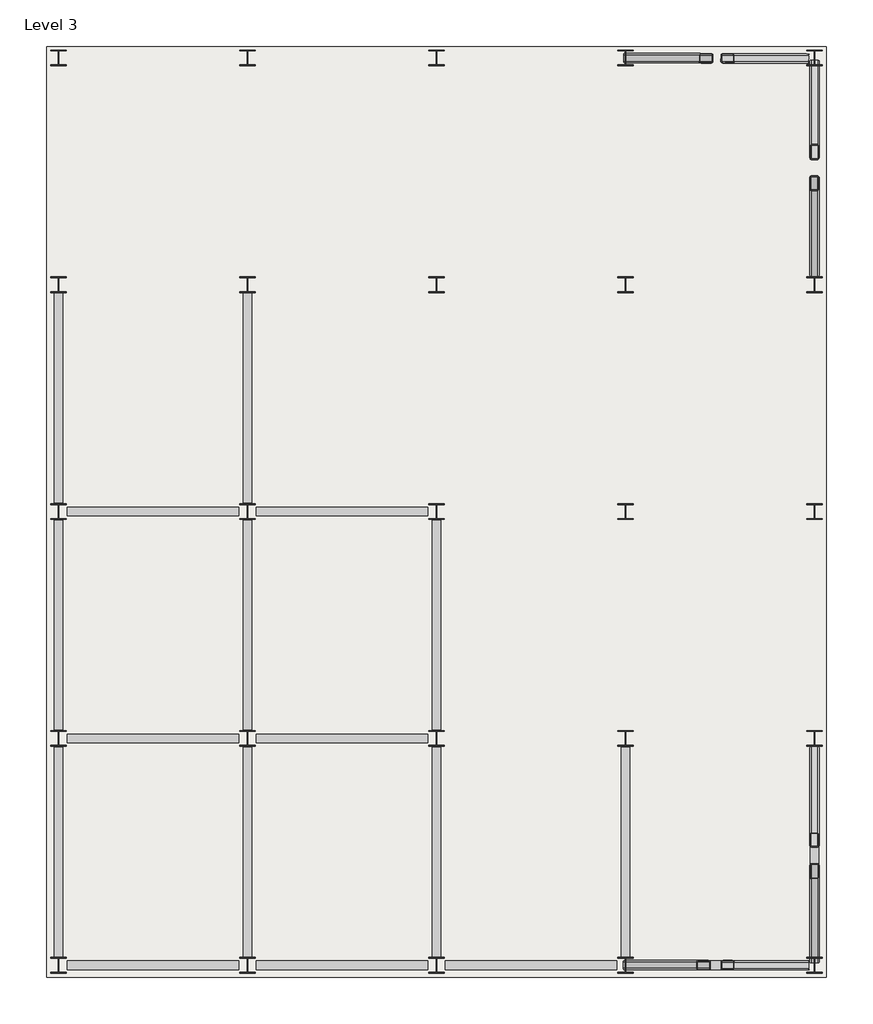
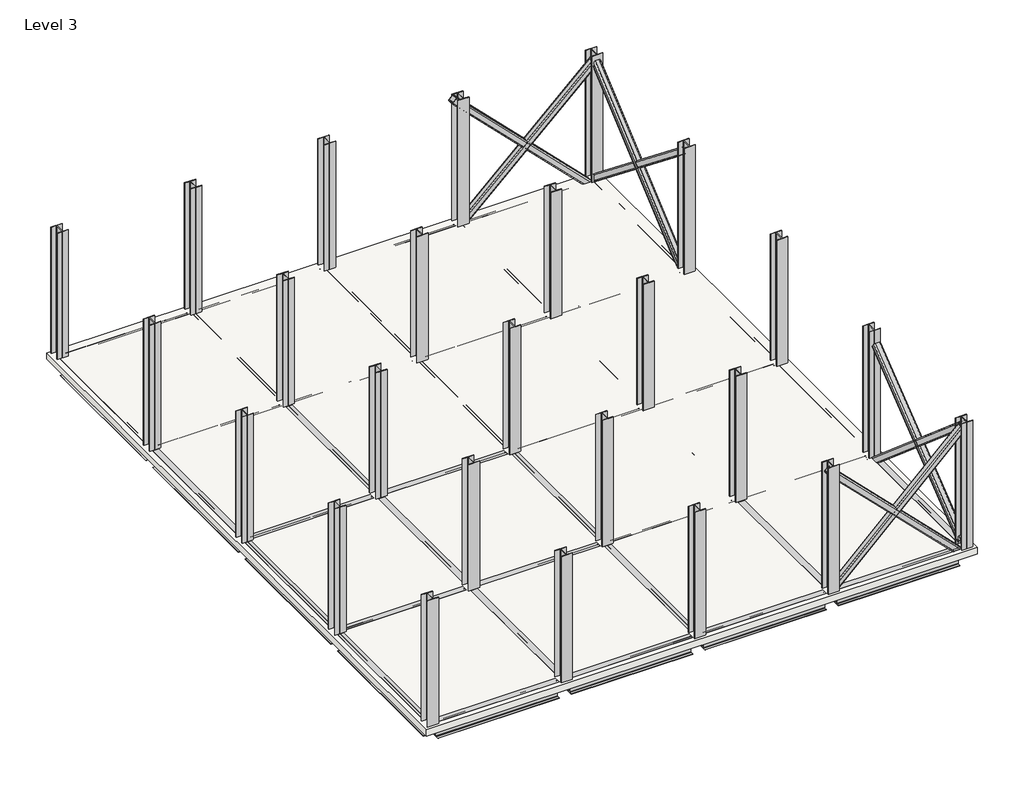
# One storey: 40 beams, 25 columns, 8 members, 1 slab.
"""IFC4 building model written with IfcOpenShell, lengths in millimetres."""

from ifc_helpers import new_model, si_unit, frame, origin, place, context, project, spatial, polyline, outline, extrude, transform, mapped, element, save
from components import w_shapes_w16x26_71b85d0e, w_shapes_w16x26_5730d789, w_shapes_column_w10x49_c7b378f5, hss_square_hss6x6x1_2_008024fe, hss_square_hss6x6x1_2_7c43692b, hss_square_hss6x6x1_2_5f011b37, hss_square_hss6x6x1_2_b9926e2d, hss_square_hss6x6x1_2_e6555cf9, hss_square_hss6x6x1_2_f7a49a43, hss_square_hss6x6x1_2_10b7330d, hss_square_hss6x6x1_2_f3b36863

model = new_model("IFC4")

# Units and contexts
model_context = context("Model", 3, world=origin())
ifc_project = project(units=[si_unit("LENGTHUNIT", "METRE", prefix="MILLI")], contexts=[model_context])

# Site, building, storey
site = spatial("IfcSite", under=ifc_project)
building = spatial("IfcBuilding", under=site)
storey = spatial("IfcBuildingStorey", under=building, Name="Level 3", Elevation=6096.0)

# Beams
placement = place(None, origin())
w_shapes_w16x26_shape = w_shapes_w16x26_71b85d0e(model_context)
element("IfcBeam", 1, ObjectType="W Shapes : W16X26", at=placement, inside=storey, context=model_context, shape_type="MappedRepresentation", body=[
    mapped(w_shapes_w16x26_shape, transform((-5883.5186598, -2213.7239423, 5896.61), x_axis=(1.0, 0.0, 0.0), y_axis=(0.0, 1.0, 0.0), z_axis=(0.0, 0.0, 1.0))),
])
element("IfcBeam", 2, ObjectType="W Shapes : W16X26", at=placement, inside=storey, context=model_context, shape_type="MappedRepresentation", body=[
    mapped(w_shapes_w16x26_shape, transform((-2835.5186598, -2213.7239423, 5896.61), x_axis=(1.0, 0.0, 0.0), y_axis=(0.0, 1.0, 0.0), z_axis=(0.0, 0.0, 1.0))),
])
element("IfcBeam", 3, ObjectType="W Shapes : W16X26", at=placement, inside=storey, context=model_context, shape_type="MappedRepresentation", body=[
    mapped(w_shapes_w16x26_shape, transform((212.4813402, -2213.7239423, 5896.61), x_axis=(1.0, 0.0, 0.0), y_axis=(0.0, 1.0, 0.0), z_axis=(0.0, 0.0, 1.0))),
])
element("IfcBeam", 4, ObjectType="W Shapes : W16X26", at=placement, inside=storey, context=model_context, shape_type="MappedRepresentation", body=[
    mapped(w_shapes_w16x26_shape, transform((3260.4813402, -2213.7239423, 5896.61), x_axis=(1.0, 0.0, 0.0), y_axis=(0.0, 1.0, 0.0), z_axis=(0.0, 0.0, 1.0))),
])
element("IfcBeam", 5, ObjectType="W Shapes : W16X26", at=placement, inside=storey, context=model_context, shape_type="MappedRepresentation", body=[
    mapped(w_shapes_w16x26_shape, transform((-5883.5186598, 1443.8760577, 5896.61), x_axis=(1.0, 0.0, 0.0), y_axis=(0.0, 1.0, 0.0), z_axis=(0.0, 0.0, 1.0))),
])
element("IfcBeam", 6, ObjectType="W Shapes : W16X26", at=placement, inside=storey, context=model_context, shape_type="MappedRepresentation", body=[
    mapped(w_shapes_w16x26_shape, transform((-2835.5186598, 1443.8760577, 5896.61), x_axis=(1.0, 0.0, 0.0), y_axis=(0.0, 1.0, 0.0), z_axis=(0.0, 0.0, 1.0))),
])
element("IfcBeam", 7, ObjectType="W Shapes : W16X26", at=placement, inside=storey, context=model_context, shape_type="MappedRepresentation", body=[
    mapped(w_shapes_w16x26_shape, transform((212.4813402, 1443.8760577, 5896.61), x_axis=(1.0, 0.0, 0.0), y_axis=(0.0, 1.0, 0.0), z_axis=(0.0, 0.0, 1.0))),
])
element("IfcBeam", 8, ObjectType="W Shapes : W16X26", at=placement, inside=storey, context=model_context, shape_type="MappedRepresentation", body=[
    mapped(w_shapes_w16x26_shape, transform((3260.4813402, 1443.8760577, 5896.61), x_axis=(1.0, 0.0, 0.0), y_axis=(0.0, 1.0, 0.0), z_axis=(0.0, 0.0, 1.0))),
])
element("IfcBeam", 9, ObjectType="W Shapes : W16X26", at=placement, inside=storey, context=model_context, shape_type="MappedRepresentation", body=[
    mapped(w_shapes_w16x26_shape, transform((-5883.5186598, 5101.4760577, 5896.61), x_axis=(1.0, 0.0, 0.0), y_axis=(0.0, 1.0, 0.0), z_axis=(0.0, 0.0, 1.0))),
])
element("IfcBeam", 10, ObjectType="W Shapes : W16X26", at=placement, inside=storey, context=model_context, shape_type="MappedRepresentation", body=[
    mapped(w_shapes_w16x26_shape, transform((-2835.5186598, 5101.4760577, 5896.61), x_axis=(1.0, 0.0, 0.0), y_axis=(0.0, 1.0, 0.0), z_axis=(0.0, 0.0, 1.0))),
])
element("IfcBeam", 11, ObjectType="W Shapes : W16X26", at=placement, inside=storey, context=model_context, shape_type="MappedRepresentation", body=[
    mapped(w_shapes_w16x26_shape, transform((212.4813402, 5101.4760577, 5896.61), x_axis=(1.0, 0.0, 0.0), y_axis=(0.0, 1.0, 0.0), z_axis=(0.0, 0.0, 1.0))),
])
element("IfcBeam", 12, ObjectType="W Shapes : W16X26", at=placement, inside=storey, context=model_context, shape_type="MappedRepresentation", body=[
    mapped(w_shapes_w16x26_shape, transform((3260.4813402, 5101.4760577, 5896.61), x_axis=(1.0, 0.0, 0.0), y_axis=(0.0, 1.0, 0.0), z_axis=(0.0, 0.0, 1.0))),
])
element("IfcBeam", 13, ObjectType="W Shapes : W16X26", at=placement, inside=storey, context=model_context, shape_type="MappedRepresentation", body=[
    mapped(w_shapes_w16x26_shape, transform((-5883.5186598, 8759.0760577, 5896.61), x_axis=(1.0, 0.0, 0.0), y_axis=(0.0, 1.0, 0.0), z_axis=(0.0, 0.0, 1.0))),
])
element("IfcBeam", 14, ObjectType="W Shapes : W16X26", at=placement, inside=storey, context=model_context, shape_type="MappedRepresentation", body=[
    mapped(w_shapes_w16x26_shape, transform((-2835.5186598, 8759.0760577, 5896.61), x_axis=(1.0, 0.0, 0.0), y_axis=(0.0, 1.0, 0.0), z_axis=(0.0, 0.0, 1.0))),
])
element("IfcBeam", 15, ObjectType="W Shapes : W16X26", at=placement, inside=storey, context=model_context, shape_type="MappedRepresentation", body=[
    mapped(w_shapes_w16x26_shape, transform((212.4813402, 8759.0760577, 5896.61), x_axis=(1.0, 0.0, 0.0), y_axis=(0.0, 1.0, 0.0), z_axis=(0.0, 0.0, 1.0))),
])
element("IfcBeam", 16, ObjectType="W Shapes : W16X26", at=placement, inside=storey, context=model_context, shape_type="MappedRepresentation", body=[
    mapped(w_shapes_w16x26_shape, transform((3260.4813402, 8759.0760577, 5896.61), x_axis=(1.0, 0.0, 0.0), y_axis=(0.0, 1.0, 0.0), z_axis=(0.0, 0.0, 1.0))),
])
element("IfcBeam", 17, ObjectType="W Shapes : W16X26", at=placement, inside=storey, context=model_context, shape_type="MappedRepresentation", body=[
    mapped(w_shapes_w16x26_shape, transform((-5883.5186598, 12416.6760577, 5896.61), x_axis=(1.0, 0.0, 0.0), y_axis=(0.0, 1.0, 0.0), z_axis=(0.0, 0.0, 1.0))),
])
element("IfcBeam", 18, ObjectType="W Shapes : W16X26", at=placement, inside=storey, context=model_context, shape_type="MappedRepresentation", body=[
    mapped(w_shapes_w16x26_shape, transform((-2835.5186598, 12416.6760577, 5896.61), x_axis=(1.0, 0.0, 0.0), y_axis=(0.0, 1.0, 0.0), z_axis=(0.0, 0.0, 1.0))),
])
element("IfcBeam", 19, ObjectType="W Shapes : W16X26", at=placement, inside=storey, context=model_context, shape_type="MappedRepresentation", body=[
    mapped(w_shapes_w16x26_shape, transform((212.4813402, 12416.6760577, 5896.61), x_axis=(1.0, 0.0, 0.0), y_axis=(0.0, 1.0, 0.0), z_axis=(0.0, 0.0, 1.0))),
])
element("IfcBeam", 20, ObjectType="W Shapes : W16X26", at=placement, inside=storey, context=model_context, shape_type="MappedRepresentation", body=[
    mapped(w_shapes_w16x26_shape, transform((3260.4813402, 12416.6760577, 5896.61), x_axis=(1.0, 0.0, 0.0), y_axis=(0.0, 1.0, 0.0), z_axis=(0.0, 0.0, 1.0))),
])
w_shapes_w16x26_2_shape = w_shapes_w16x26_5730d789(model_context)
element("IfcBeam", 21, ObjectType="W Shapes : W16X26", at=placement, inside=storey, context=model_context, shape_type="MappedRepresentation", body=[
    mapped(w_shapes_w16x26_2_shape, transform((4784.4813402, 10587.8760577, 5896.61), x_axis=(0.0, -1.0, 0.0), y_axis=(1.0, 0.0, 0.0), z_axis=(0.0, 0.0, 1.0))),
])
element("IfcBeam", 22, ObjectType="W Shapes : W16X26", at=placement, inside=storey, context=model_context, shape_type="MappedRepresentation", body=[
    mapped(w_shapes_w16x26_2_shape, transform((4784.4813402, 6930.2760577, 5896.61), x_axis=(0.0, -1.0, 0.0), y_axis=(1.0, 0.0, 0.0), z_axis=(0.0, 0.0, 1.0))),
])
element("IfcBeam", 23, ObjectType="W Shapes : W16X26", at=placement, inside=storey, context=model_context, shape_type="MappedRepresentation", body=[
    mapped(w_shapes_w16x26_2_shape, transform((4784.4813402, 3272.6760577, 5896.61), x_axis=(0.0, -1.0, 0.0), y_axis=(1.0, 0.0, 0.0), z_axis=(0.0, 0.0, 1.0))),
])
element("IfcBeam", 24, ObjectType="W Shapes : W16X26", at=placement, inside=storey, context=model_context, shape_type="MappedRepresentation", body=[
    mapped(w_shapes_w16x26_2_shape, transform((4784.4813402, -384.9239423, 5896.61), x_axis=(0.0, -1.0, 0.0), y_axis=(1.0, 0.0, 0.0), z_axis=(0.0, 0.0, 1.0))),
])
element("IfcBeam", 25, ObjectType="W Shapes : W16X26", at=placement, inside=storey, context=model_context, shape_type="MappedRepresentation", body=[
    mapped(w_shapes_w16x26_2_shape, transform((1736.4813402, 10587.8760577, 5896.61), x_axis=(0.0, -1.0, 0.0), y_axis=(1.0, 0.0, 0.0), z_axis=(0.0, 0.0, 1.0))),
])
element("IfcBeam", 26, ObjectType="W Shapes : W16X26", at=placement, inside=storey, context=model_context, shape_type="MappedRepresentation", body=[
    mapped(w_shapes_w16x26_2_shape, transform((1736.4813402, 6930.2760577, 5896.61), x_axis=(0.0, -1.0, 0.0), y_axis=(1.0, 0.0, 0.0), z_axis=(0.0, 0.0, 1.0))),
])
element("IfcBeam", 27, ObjectType="W Shapes : W16X26", at=placement, inside=storey, context=model_context, shape_type="MappedRepresentation", body=[
    mapped(w_shapes_w16x26_2_shape, transform((1736.4813402, 3272.6760577, 5896.61), x_axis=(0.0, -1.0, 0.0), y_axis=(1.0, 0.0, 0.0), z_axis=(0.0, 0.0, 1.0))),
])
element("IfcBeam", 28, ObjectType="W Shapes : W16X26", at=placement, inside=storey, context=model_context, shape_type="MappedRepresentation", body=[
    mapped(w_shapes_w16x26_2_shape, transform((1736.4813402, -384.9239423, 5896.61), x_axis=(0.0, -1.0, 0.0), y_axis=(1.0, 0.0, 0.0), z_axis=(0.0, 0.0, 1.0))),
])
element("IfcBeam", 29, ObjectType="W Shapes : W16X26", at=placement, inside=storey, context=model_context, shape_type="MappedRepresentation", body=[
    mapped(w_shapes_w16x26_2_shape, transform((-1311.5186598, 10587.8760577, 5896.61), x_axis=(0.0, -1.0, 0.0), y_axis=(1.0, 0.0, 0.0), z_axis=(0.0, 0.0, 1.0))),
])
element("IfcBeam", 30, ObjectType="W Shapes : W16X26", at=placement, inside=storey, context=model_context, shape_type="MappedRepresentation", body=[
    mapped(w_shapes_w16x26_2_shape, transform((-1311.5186598, 6930.2760577, 5896.61), x_axis=(0.0, -1.0, 0.0), y_axis=(1.0, 0.0, 0.0), z_axis=(0.0, 0.0, 1.0))),
])
element("IfcBeam", 31, ObjectType="W Shapes : W16X26", at=placement, inside=storey, context=model_context, shape_type="MappedRepresentation", body=[
    mapped(w_shapes_w16x26_2_shape, transform((-1311.5186598, 3272.6760577, 5896.61), x_axis=(0.0, -1.0, 0.0), y_axis=(1.0, 0.0, 0.0), z_axis=(0.0, 0.0, 1.0))),
])
element("IfcBeam", 32, ObjectType="W Shapes : W16X26", at=placement, inside=storey, context=model_context, shape_type="MappedRepresentation", body=[
    mapped(w_shapes_w16x26_2_shape, transform((-1311.5186598, -384.9239423, 5896.61), x_axis=(0.0, -1.0, 0.0), y_axis=(1.0, 0.0, 0.0), z_axis=(0.0, 0.0, 1.0))),
])
element("IfcBeam", 33, ObjectType="W Shapes : W16X26", at=placement, inside=storey, context=model_context, shape_type="MappedRepresentation", body=[
    mapped(w_shapes_w16x26_2_shape, transform((-4359.5186598, 10587.8760577, 5896.61), x_axis=(0.0, -1.0, 0.0), y_axis=(1.0, 0.0, 0.0), z_axis=(0.0, 0.0, 1.0))),
])
element("IfcBeam", 34, ObjectType="W Shapes : W16X26", at=placement, inside=storey, context=model_context, shape_type="MappedRepresentation", body=[
    mapped(w_shapes_w16x26_2_shape, transform((-4359.5186598, 6930.2760577, 5896.61), x_axis=(0.0, -1.0, 0.0), y_axis=(1.0, 0.0, 0.0), z_axis=(0.0, 0.0, 1.0))),
])
element("IfcBeam", 35, ObjectType="W Shapes : W16X26", at=placement, inside=storey, context=model_context, shape_type="MappedRepresentation", body=[
    mapped(w_shapes_w16x26_2_shape, transform((-4359.5186598, 3272.6760577, 5896.61), x_axis=(0.0, -1.0, 0.0), y_axis=(1.0, 0.0, 0.0), z_axis=(0.0, 0.0, 1.0))),
])
element("IfcBeam", 36, ObjectType="W Shapes : W16X26", at=placement, inside=storey, context=model_context, shape_type="MappedRepresentation", body=[
    mapped(w_shapes_w16x26_2_shape, transform((-4359.5186598, -384.9239423, 5896.61), x_axis=(0.0, -1.0, 0.0), y_axis=(1.0, 0.0, 0.0), z_axis=(0.0, 0.0, 1.0))),
])
element("IfcBeam", 37, ObjectType="W Shapes : W16X26", at=placement, inside=storey, context=model_context, shape_type="MappedRepresentation", body=[
    mapped(w_shapes_w16x26_2_shape, transform((-7407.5186598, 10587.8760577, 5896.61), x_axis=(0.0, -1.0, 0.0), y_axis=(1.0, 0.0, 0.0), z_axis=(0.0, 0.0, 1.0))),
])
element("IfcBeam", 38, ObjectType="W Shapes : W16X26", at=placement, inside=storey, context=model_context, shape_type="MappedRepresentation", body=[
    mapped(w_shapes_w16x26_2_shape, transform((-7407.5186598, 6930.2760577, 5896.61), x_axis=(0.0, -1.0, 0.0), y_axis=(1.0, 0.0, 0.0), z_axis=(0.0, 0.0, 1.0))),
])
element("IfcBeam", 39, ObjectType="W Shapes : W16X26", at=placement, inside=storey, context=model_context, shape_type="MappedRepresentation", body=[
    mapped(w_shapes_w16x26_2_shape, transform((-7407.5186598, 3272.6760577, 5896.61), x_axis=(0.0, -1.0, 0.0), y_axis=(1.0, 0.0, 0.0), z_axis=(0.0, 0.0, 1.0))),
])
element("IfcBeam", 40, ObjectType="W Shapes : W16X26", at=placement, inside=storey, context=model_context, shape_type="MappedRepresentation", body=[
    mapped(w_shapes_w16x26_2_shape, transform((-7407.5186598, -384.9239423, 5896.61), x_axis=(0.0, -1.0, 0.0), y_axis=(1.0, 0.0, 0.0), z_axis=(0.0, 0.0, 1.0))),
])

# Columns
w_shapes_column_w10x49_shape = w_shapes_column_w10x49_c7b378f5(model_context)
element("IfcColumn", 41, ObjectType="W Shapes-Column : W10X49", at=placement, inside=storey, context=model_context, shape_type="MappedRepresentation", body=[
    mapped(w_shapes_column_w10x49_shape, transform((4784.4813402, -2213.7239423, 0.0), x_axis=(1.0, 0.0, 0.0), y_axis=(0.0, 1.0, 0.0), z_axis=(0.0, 0.0, 1.0))),
])
element("IfcColumn", 42, ObjectType="W Shapes-Column : W10X49", at=placement, inside=storey, context=model_context, shape_type="MappedRepresentation", body=[
    mapped(w_shapes_column_w10x49_shape, transform((1736.4813402, -2213.7239423, 0.0), x_axis=(1.0, 0.0, 0.0), y_axis=(0.0, 1.0, 0.0), z_axis=(0.0, 0.0, 1.0))),
])
element("IfcColumn", 43, ObjectType="W Shapes-Column : W10X49", at=placement, inside=storey, context=model_context, shape_type="MappedRepresentation", body=[
    mapped(w_shapes_column_w10x49_shape, transform((-1311.5186598, -2213.7239423, 0.0), x_axis=(1.0, 0.0, 0.0), y_axis=(0.0, 1.0, 0.0), z_axis=(0.0, 0.0, 1.0))),
])
element("IfcColumn", 44, ObjectType="W Shapes-Column : W10X49", at=placement, inside=storey, context=model_context, shape_type="MappedRepresentation", body=[
    mapped(w_shapes_column_w10x49_shape, transform((-4359.5186598, -2213.7239423, 0.0), x_axis=(1.0, 0.0, 0.0), y_axis=(0.0, 1.0, 0.0), z_axis=(0.0, 0.0, 1.0))),
])
element("IfcColumn", 45, ObjectType="W Shapes-Column : W10X49", at=placement, inside=storey, context=model_context, shape_type="MappedRepresentation", body=[
    mapped(w_shapes_column_w10x49_shape, transform((-7407.5186598, -2213.7239423, 0.0), x_axis=(1.0, 0.0, 0.0), y_axis=(0.0, 1.0, 0.0), z_axis=(0.0, 0.0, 1.0))),
])
element("IfcColumn", 46, ObjectType="W Shapes-Column : W10X49", at=placement, inside=storey, context=model_context, shape_type="MappedRepresentation", body=[
    mapped(w_shapes_column_w10x49_shape, transform((4784.4813402, 1443.8760577, 0.0), x_axis=(1.0, 0.0, 0.0), y_axis=(0.0, 1.0, 0.0), z_axis=(0.0, 0.0, 1.0))),
])
element("IfcColumn", 47, ObjectType="W Shapes-Column : W10X49", at=placement, inside=storey, context=model_context, shape_type="MappedRepresentation", body=[
    mapped(w_shapes_column_w10x49_shape, transform((4784.4813402, 5101.4760577, 0.0), x_axis=(1.0, 0.0, 0.0), y_axis=(0.0, 1.0, 0.0), z_axis=(0.0, 0.0, 1.0))),
])
element("IfcColumn", 48, ObjectType="W Shapes-Column : W10X49", at=placement, inside=storey, context=model_context, shape_type="MappedRepresentation", body=[
    mapped(w_shapes_column_w10x49_shape, transform((4784.4813402, 8759.0760577, 0.0), x_axis=(1.0, 0.0, 0.0), y_axis=(0.0, 1.0, 0.0), z_axis=(0.0, 0.0, 1.0))),
])
element("IfcColumn", 49, ObjectType="W Shapes-Column : W10X49", at=placement, inside=storey, context=model_context, shape_type="MappedRepresentation", body=[
    mapped(w_shapes_column_w10x49_shape, transform((4784.4813402, 12416.6760577, 0.0), x_axis=(1.0, 0.0, 0.0), y_axis=(0.0, 1.0, 0.0), z_axis=(0.0, 0.0, 1.0))),
])
element("IfcColumn", 50, ObjectType="W Shapes-Column : W10X49", at=placement, inside=storey, context=model_context, shape_type="MappedRepresentation", body=[
    mapped(w_shapes_column_w10x49_shape, transform((1736.4813402, 1443.8760577, 0.0), x_axis=(1.0, 0.0, 0.0), y_axis=(0.0, 1.0, 0.0), z_axis=(0.0, 0.0, 1.0))),
])
element("IfcColumn", 51, ObjectType="W Shapes-Column : W10X49", at=placement, inside=storey, context=model_context, shape_type="MappedRepresentation", body=[
    mapped(w_shapes_column_w10x49_shape, transform((-1311.5186598, 1443.8760577, 0.0), x_axis=(1.0, 0.0, 0.0), y_axis=(0.0, 1.0, 0.0), z_axis=(0.0, 0.0, 1.0))),
])
element("IfcColumn", 52, ObjectType="W Shapes-Column : W10X49", at=placement, inside=storey, context=model_context, shape_type="MappedRepresentation", body=[
    mapped(w_shapes_column_w10x49_shape, transform((-4359.5186598, 1443.8760577, 0.0), x_axis=(1.0, 0.0, 0.0), y_axis=(0.0, 1.0, 0.0), z_axis=(0.0, 0.0, 1.0))),
])
element("IfcColumn", 53, ObjectType="W Shapes-Column : W10X49", at=placement, inside=storey, context=model_context, shape_type="MappedRepresentation", body=[
    mapped(w_shapes_column_w10x49_shape, transform((-7407.5186598, 1443.8760577, 0.0), x_axis=(1.0, 0.0, 0.0), y_axis=(0.0, 1.0, 0.0), z_axis=(0.0, 0.0, 1.0))),
])
element("IfcColumn", 54, ObjectType="W Shapes-Column : W10X49", at=placement, inside=storey, context=model_context, shape_type="MappedRepresentation", body=[
    mapped(w_shapes_column_w10x49_shape, transform((1736.4813402, 5101.4760577, 0.0), x_axis=(1.0, 0.0, 0.0), y_axis=(0.0, 1.0, 0.0), z_axis=(0.0, 0.0, 1.0))),
])
element("IfcColumn", 55, ObjectType="W Shapes-Column : W10X49", at=placement, inside=storey, context=model_context, shape_type="MappedRepresentation", body=[
    mapped(w_shapes_column_w10x49_shape, transform((-1311.5186598, 5101.4760577, 0.0), x_axis=(1.0, 0.0, 0.0), y_axis=(0.0, 1.0, 0.0), z_axis=(0.0, 0.0, 1.0))),
])
element("IfcColumn", 56, ObjectType="W Shapes-Column : W10X49", at=placement, inside=storey, context=model_context, shape_type="MappedRepresentation", body=[
    mapped(w_shapes_column_w10x49_shape, transform((-4359.5186598, 5101.4760577, 0.0), x_axis=(1.0, 0.0, 0.0), y_axis=(0.0, 1.0, 0.0), z_axis=(0.0, 0.0, 1.0))),
])
element("IfcColumn", 57, ObjectType="W Shapes-Column : W10X49", at=placement, inside=storey, context=model_context, shape_type="MappedRepresentation", body=[
    mapped(w_shapes_column_w10x49_shape, transform((-7407.5186598, 5101.4760577, 0.0), x_axis=(1.0, 0.0, 0.0), y_axis=(0.0, 1.0, 0.0), z_axis=(0.0, 0.0, 1.0))),
])
element("IfcColumn", 58, ObjectType="W Shapes-Column : W10X49", at=placement, inside=storey, context=model_context, shape_type="MappedRepresentation", body=[
    mapped(w_shapes_column_w10x49_shape, transform((1736.4813402, 8759.0760577, 0.0), x_axis=(1.0, 0.0, 0.0), y_axis=(0.0, 1.0, 0.0), z_axis=(0.0, 0.0, 1.0))),
])
element("IfcColumn", 59, ObjectType="W Shapes-Column : W10X49", at=placement, inside=storey, context=model_context, shape_type="MappedRepresentation", body=[
    mapped(w_shapes_column_w10x49_shape, transform((-1311.5186598, 8759.0760577, 0.0), x_axis=(1.0, 0.0, 0.0), y_axis=(0.0, 1.0, 0.0), z_axis=(0.0, 0.0, 1.0))),
])
element("IfcColumn", 60, ObjectType="W Shapes-Column : W10X49", at=placement, inside=storey, context=model_context, shape_type="MappedRepresentation", body=[
    mapped(w_shapes_column_w10x49_shape, transform((-4359.5186598, 8759.0760577, 0.0), x_axis=(1.0, 0.0, 0.0), y_axis=(0.0, 1.0, 0.0), z_axis=(0.0, 0.0, 1.0))),
])
element("IfcColumn", 61, ObjectType="W Shapes-Column : W10X49", at=placement, inside=storey, context=model_context, shape_type="MappedRepresentation", body=[
    mapped(w_shapes_column_w10x49_shape, transform((-7407.5186598, 8759.0760577, 0.0), x_axis=(1.0, 0.0, 0.0), y_axis=(0.0, 1.0, 0.0), z_axis=(0.0, 0.0, 1.0))),
])
element("IfcColumn", 62, ObjectType="W Shapes-Column : W10X49", at=placement, inside=storey, context=model_context, shape_type="MappedRepresentation", body=[
    mapped(w_shapes_column_w10x49_shape, transform((1736.4813402, 12416.6760577, 0.0), x_axis=(1.0, 0.0, 0.0), y_axis=(0.0, 1.0, 0.0), z_axis=(0.0, 0.0, 1.0))),
])
element("IfcColumn", 63, ObjectType="W Shapes-Column : W10X49", at=placement, inside=storey, context=model_context, shape_type="MappedRepresentation", body=[
    mapped(w_shapes_column_w10x49_shape, transform((-1311.5186598, 12416.6760577, 0.0), x_axis=(1.0, 0.0, 0.0), y_axis=(0.0, 1.0, 0.0), z_axis=(0.0, 0.0, 1.0))),
])
element("IfcColumn", 64, ObjectType="W Shapes-Column : W10X49", at=placement, inside=storey, context=model_context, shape_type="MappedRepresentation", body=[
    mapped(w_shapes_column_w10x49_shape, transform((-4359.5186598, 12416.6760577, 0.0), x_axis=(1.0, 0.0, 0.0), y_axis=(0.0, 1.0, 0.0), z_axis=(0.0, 0.0, 1.0))),
])
element("IfcColumn", 65, ObjectType="W Shapes-Column : W10X49", at=placement, inside=storey, context=model_context, shape_type="MappedRepresentation", body=[
    mapped(w_shapes_column_w10x49_shape, transform((-7407.5186598, 12416.6760577, 0.0), x_axis=(1.0, 0.0, 0.0), y_axis=(0.0, 1.0, 0.0), z_axis=(0.0, 0.0, 1.0))),
])

# Members
hss_square_hss6x6x1_2_shape = hss_square_hss6x6x1_2_008024fe(model_context)
element("IfcMember", 66, ObjectType="HSS Square : HSS6X6X1/2", at=placement, inside=storey, context=model_context, shape_type="MappedRepresentation", body=[
    mapped(hss_square_hss6x6x1_2_shape, transform((4784.4813402, 10587.8760577, 7543.8), x_axis=(0.0, 0.7840458244617616, -0.6207029443655613), y_axis=(-1.0000000000000002, 0.0, 0.0), z_axis=(0.0, 0.6207029443655613, 0.7840458244617616))),
])
hss_square_hss6x6x1_2_2_shape = hss_square_hss6x6x1_2_7c43692b(model_context)
element("IfcMember", 67, ObjectType="HSS Square : HSS6X6X1/2", at=placement, inside=storey, context=model_context, shape_type="MappedRepresentation", body=[
    mapped(hss_square_hss6x6x1_2_2_shape, transform((4784.4813402, 10587.8760577, 7460.1631022), x_axis=(0.0, -0.760075346032819, -0.6498349547024159), y_axis=(1.0000000000000002, 0.0, 0.0), z_axis=(0.0, -0.6498349547024159, 0.760075346032819))),
])
hss_square_hss6x6x1_2_3_shape = hss_square_hss6x6x1_2_5f011b37(model_context)
element("IfcMember", 68, ObjectType="HSS Square : HSS6X6X1/2", at=placement, inside=storey, context=model_context, shape_type="MappedRepresentation", body=[
    mapped(hss_square_hss6x6x1_2_3_shape, transform((4784.4813402, -384.9239423, 7460.1631022), x_axis=(0.0, 0.760075346032819, -0.6498349547024159), y_axis=(-1.0000000000000002, 0.0, 0.0), z_axis=(0.0, 0.6498349547024159, 0.760075346032819))),
])
hss_square_hss6x6x1_2_4_shape = hss_square_hss6x6x1_2_b9926e2d(model_context)
element("IfcMember", 69, ObjectType="HSS Square : HSS6X6X1/2", at=placement, inside=storey, context=model_context, shape_type="MappedRepresentation", body=[
    mapped(hss_square_hss6x6x1_2_4_shape, transform((4784.4813402, -384.9239423, 7543.8), x_axis=(0.0, -0.7840458244617616, -0.6207029443655613), y_axis=(1.0000000000000002, 0.0, 0.0), z_axis=(0.0, -0.6207029443655613, 0.7840458244617616))),
])
hss_square_hss6x6x1_2_5_shape = hss_square_hss6x6x1_2_e6555cf9(model_context)
element("IfcMember", 70, ObjectType="HSS Square : HSS6X6X1/2", at=placement, inside=storey, context=model_context, shape_type="MappedRepresentation", body=[
    mapped(hss_square_hss6x6x1_2_5_shape, transform((3168.0352384, -2213.7239423, 7461.8521986), x_axis=(-0.718393447364439, 0.0, -0.6956370136672122), y_axis=(0.0, -1.0000000000000002, 0.0), z_axis=(-0.6956370136672122, 0.0, 0.718393447364439))),
])
hss_square_hss6x6x1_2_6_shape = hss_square_hss6x6x1_2_f7a49a43(model_context)
element("IfcMember", 71, ObjectType="HSS Square : HSS6X6X1/2", at=placement, inside=storey, context=model_context, shape_type="MappedRepresentation", body=[
    mapped(hss_square_hss6x6x1_2_6_shape, transform((3260.4813402, -2213.7239423, 7420.61), x_axis=(0.7071067811865474, 0.0, -0.7071067811865478), y_axis=(0.0, 1.0000000000000002, 0.0), z_axis=(0.7071067811865478, 0.0, 0.7071067811865474))),
])
hss_square_hss6x6x1_2_7_shape = hss_square_hss6x6x1_2_10b7330d(model_context)
element("IfcMember", 72, ObjectType="HSS Square : HSS6X6X1/2", at=placement, inside=storey, context=model_context, shape_type="MappedRepresentation", body=[
    mapped(hss_square_hss6x6x1_2_7_shape, transform((3168.0352384, 12409.9819642, 7420.61), x_axis=(-0.727603572033317, 0.003013182054487478, -0.685991226400356), y_axis=(-0.004141205915939177, -0.9999914251700174, 0.0), z_axis=(-0.6859853441422199, 0.0028408309250506723, 0.7276098111637418))),
])
hss_square_hss6x6x1_2_8_shape = hss_square_hss6x6x1_2_f3b36863(model_context)
element("IfcMember", 73, ObjectType="HSS Square : HSS6X6X1/2", at=placement, inside=storey, context=model_context, shape_type="MappedRepresentation", body=[
    mapped(hss_square_hss6x6x1_2_8_shape, transform((3260.4813402, 12409.9819642, 7420.61), x_axis=(0.7071033705496138, -0.0031059160887349836, -0.7071033705496146), y_axis=(0.004392407470180803, 0.9999903533317791, 0.0), z_axis=(0.7070965493580008, -0.0031058861269913462, 0.7071101918070299))),
])

# Slab
element("IfcSlab", 74, ObjectType="6\" Foundation Slab", at=placement, inside=storey, context=model_context, shape_type="SweptSolid", body=[
    extrude(outline(polyline([(4974.3230176, 12600.4819642), (4974.3230176, -2410.9180358), (-7598.6769824, -2410.9180358), (-7598.6769824, 12600.4819642), (4974.3230176, 12600.4819642)])), frame((0.0, 0.0, 5943.6), z_axis=(0.0, 0.0, 1.0), x_axis=(1.0, 0.0, 0.0)), (0.0, 0.0, 1.0), 152.4),
])

save(model, "model.ifc")

# Revit data of these elements
# Type "W Shapes : W16X26"
#   Section Name Key = "W16x26"
#   Assembly Code = "B10"
#   Width = 5.500"
#   Web Thickness = 0.250"
#   Web Fillet = 0.402"
#   Warping Constant = 565.00 in⁶
#   Torsional Moment of Inertia = 0.262 in⁴
#   Section Area = 7.68 in²
#   Plastic Modulus weak axis = 5.48 in³
#   Plastic Modulus strong axis = 44.20 in³
#   Perimeter = 52.20 ft²/ft
#   Nominal Weight = 26.00 lbf/ft
#   Moment of Inertia weak axis = 9.59 in⁴
#   Moment of Inertia strong axis = 301.00 in⁴
#   Height = 15.700"
#   Flange Thickness = 0.345"
#   Elastic Modulus weak axis = 3.49 in³
#   Elastic Modulus strong axis = 38.40 in³
#   Centroid Vertical = 7.850"
#   Centroid Horizontal = 2.750"
#   Bolt Spacing = 0' - 3 1/2"
#   Length [instance default] = 5' - 0"
#   Structural Material [instance default] = Steel ASTM A992
#   Principal Axes Angle = 0
# Type "W Shapes-Column : W10X49"
#   Section Name Key = "W10x49"
#   Assembly Code = "B10"
#   Width = 10.000"
#   Web Thickness = 0.340"
#   Web Fillet = 0.500"
#   Warping Constant = 2070.00 in⁶
#   Torsional Moment of Inertia = 1.39 in⁴
#   Section Area = 14.40 in²
#   Plastic Modulus weak axis = 28.30 in³
#   Plastic Modulus strong axis = 60.40 in³
#   Perimeter = 58.50 ft²/ft
#   Nominal Weight = 49.00 lbf/ft
#   Moment of Inertia weak axis = 93.40 in⁴
#   Moment of Inertia strong axis = 272.00 in⁴
#   Height = 10.000"
#   Flange Thickness = 0.560"
#   Elastic Modulus weak axis = 18.70 in³
#   Elastic Modulus strong axis = 54.60 in³
#   Centroid Vertical = 5.000"
#   Centroid Horizontal = 5.000"
#   Bolt Spacing = 0' - 5 1/2"
#   Structural Material [instance default] = Steel ASTM A992
#   Principal Axes Angle = 0
# Type "HSS Square : HSS6X6X1/2"
#   Section Name Key = "HSS 6X6X1/2"
#   Assembly Code = "B10"
#   Width = 6.000"
#   Wall Nominal Thickness = 0.500"
#   Wall Design Thickness = 0.465"
#   Torsional Moment of Inertia = 81.10 in⁴
#   Torsional Modulus = 28.10 in³
#   Section Area = 9.74 in²
#   Plastic Modulus weak axis = 19.80 in³
#   Plastic Modulus strong axis = 19.80 in³
#   Outer Fillet = 1.000"
#   Nominal Weight = 35.24 lbf/ft
#   Moment of Inertia weak axis = 48.30 in⁴
#   Moment of Inertia strong axis = 48.30 in⁴
#   Inner Fillet = 0.500"
#   Height = 6.000"
#   Elastic Modulus weak axis = 16.10 in³
#   Elastic Modulus strong axis = 16.10 in³
#   Centroid Vertical = 3.000"
#   Centroid Horizontal = 3.000"
#   Length [instance default] = 5' - 0"
#   Structural Material [instance default] = Steel ASTM A500, Grade B, Rectangular and Square
#   Principal Axes Angle = 0
# Type "6\" Foundation Slab"
#   Layers, outside or top first: 0' - 6" "Concrete, Cast-in-Place gray" (function 1)
# Elements 1, 2, 3, 4, 5, 6, 7, 8, 9, 10, 11, 12, 13, 14, 15, 16, 17, 18, 19, 20, 21, 22, 23, 24, 25, 26, 27, 28, 29, 30, 31, 32, 33, 34, 35, 36, 37, 38, 39, 40 (IfcBeam, "W Shapes : W16X26")
#   Comments = ""
#   Structural Material = Steel ASTM A992
#   Phase Created = New Construction
#   Materials on its faces: "Steel ASTM A992"
# Elements 41, 42, 43, 44, 45, 46, 47, 48, 49, 50, 51, 52, 53, 54, 55, 56, 57, 58, 59, 60, 61, 62, 63, 64, 65 (IfcColumn, "W Shapes-Column : W10X49")
#   Structural Material = Steel ASTM A992
#   Phase Created = New Construction
#   Materials on its faces: "Steel ASTM A992"
# Elements 66, 67, 68, 69, 70, 71, 72, 73 (IfcMember, "HSS Square : HSS6X6X1/2")
#   Comments = ""
#   Structural Material = Steel ASTM A992
#   Phase Created = New Construction
#   Materials on its faces: "Steel ASTM A992"
# Element 74 (IfcSlab, "6\" Foundation Slab")
#   Height Offset From Level = 0' - 0"
#   built-in parameter 1001954 = 1
#   Phase Created = New Construction
#   Materials on its faces: "Concrete, Cast-in-Place gray"
# Materials
#   "Steel ASTM A992": class "Metal", colour RGB 199 199 199, transparency 0, Description = "Structural steel 50ksi", Cost = 0
#   "Steel ASTM A500, Grade B, Rectangular and Square": class "Metal", colour RGB 199 199 199, transparency 0, Description = "Carbon steel", Cost = 0
#   "Concrete, Cast-in-Place gray": class "Concrete", colour RGB 192 192 192, transparency 0, Description = "Cast-in-place concrete", Cost = 0
